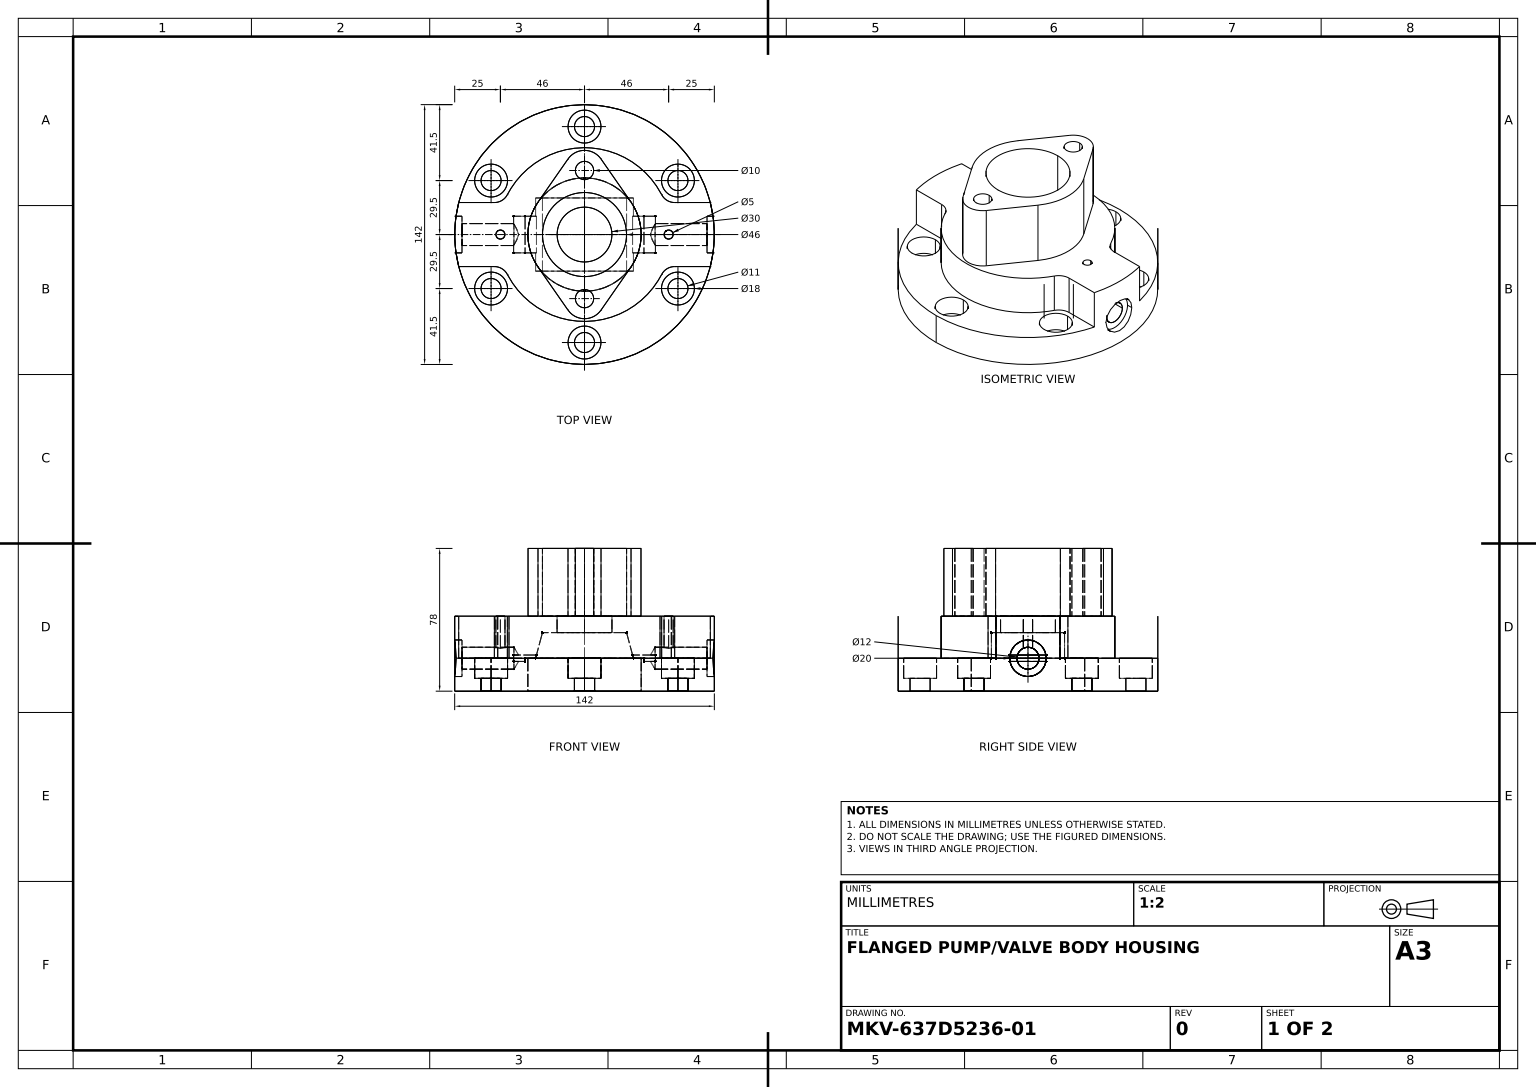
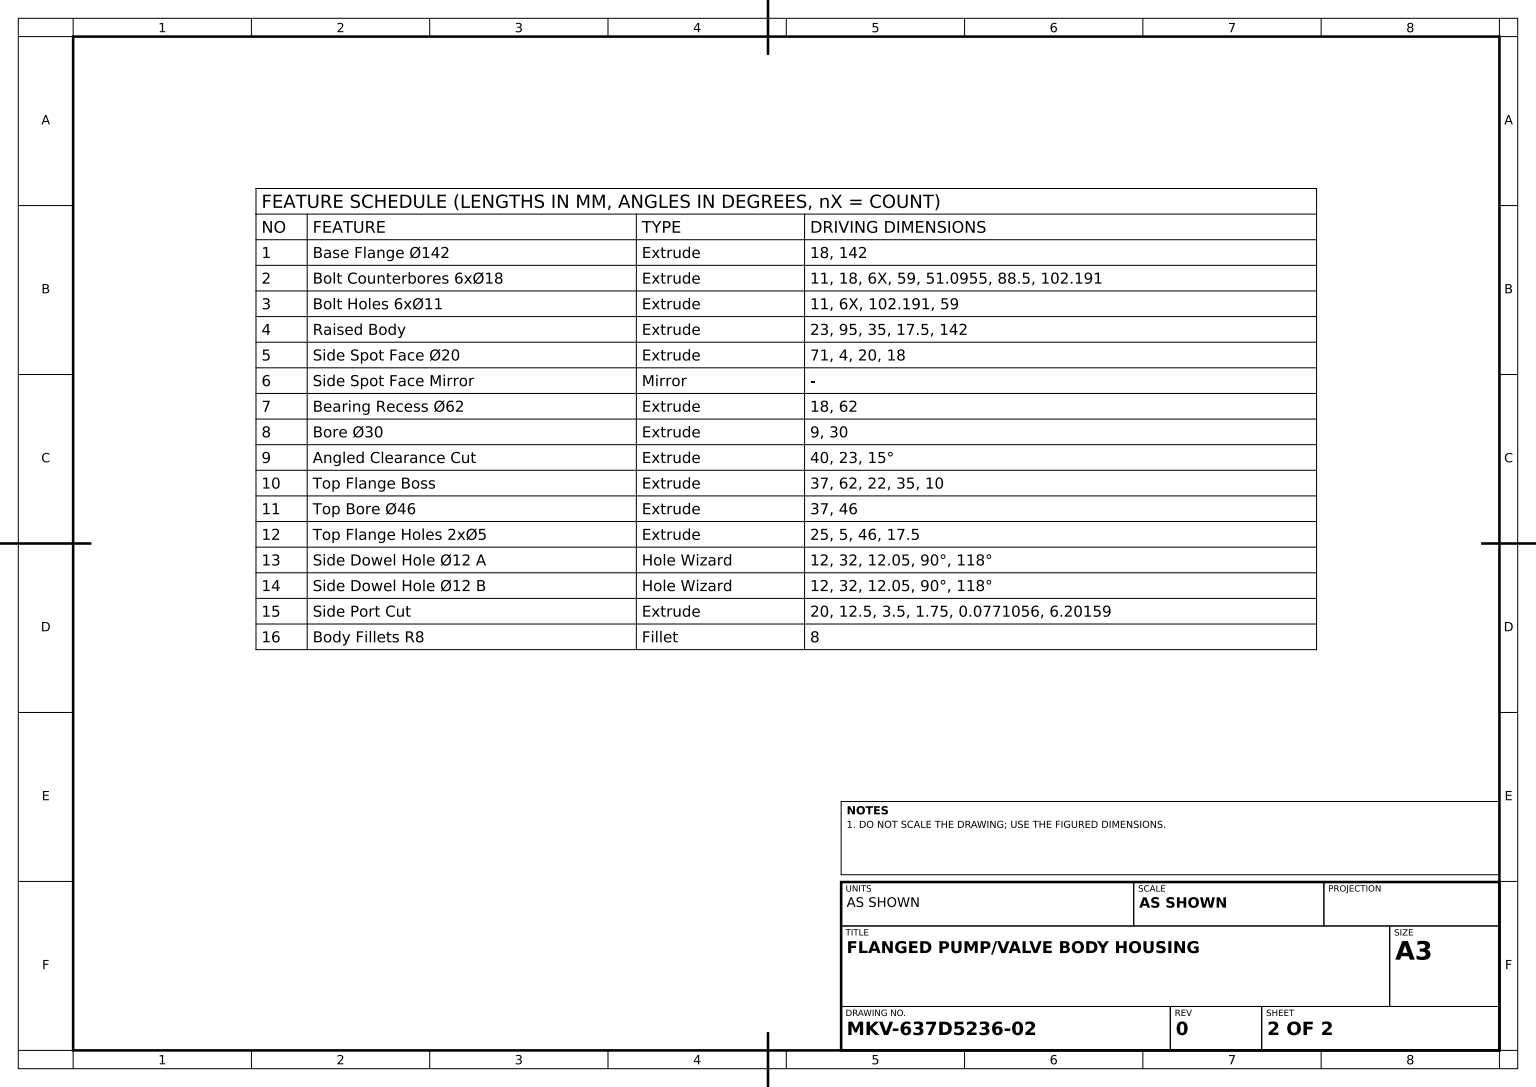
from build123d import *
from build123d.topology import SkipClean

# Parameters (mm, degrees)
BASE_FLANGE_SKETCH_R             = 71
BASE_FLANGE_142_DEPTH            = 18
COUNTERBORE_SKETCH_R             = 9
BOLT_COUNTERBORES_6X_18_DEPTH    = 11
BOLT_HOLE_SKETCH_R               = 5.5
BOLT_HOLES_6X_11_DEPTH           = 11
RAISED_BODY_DEPTH                = 23
SIDE_SPOT_FACE_SKETCH_R          = 10
SIDE_SPOT_FACE_20_DEPTH          = 4
BEARING_RECESS_SKETCH_R          = 31
BEARING_RECESS_62_DEPTH          = 18
BORE_30_SKETCH_R                 = 15
BORE_30_DEPTH                    = 9
ANGLED_CLEARANCE_CUT_DEPTH       = 20
TOP_FLANGE_BOSS_SKETCH_R         = 5
TOP_FLANGE_BOSS_DEPTH            = 37
TOP_BORE_SKETCH_R                = 23
TOP_BORE_46_DEPTH                = 37
TOP_FLANGE_HOLES_SKETCH_R        = 2.5
TOP_FLANGE_HOLES_2X_5_DEPTH      = 25
SIDE_DOWEL_HOLE_12_A_D           = 12
SIDE_DOWEL_HOLE_12_A_DEPTH       = 28.394836286
SIDE_DOWEL_HOLE_12_A_CSINK_D     = 12.05
SIDE_DOWEL_HOLE_12_A_CSINK_ANGLE = 90
SIDE_DOWEL_HOLE_12_A_TIP         = 3.605163714
SIDE_DOWEL_HOLE_12_B_D           = 12
SIDE_DOWEL_HOLE_12_B_DEPTH       = 28.394836286
SIDE_DOWEL_HOLE_12_B_CSINK_D     = 12.05
SIDE_DOWEL_HOLE_12_B_CSINK_ANGLE = 90
SIDE_DOWEL_HOLE_12_B_TIP         = 3.605163714
SIDE_PORT_CUT_DEPTH              = 10
BODY_FILLETS_R8_R                = 8


with BuildPart() as part:
    # Base Flange Sketch → Base Flange Ø142 (new body)
    with BuildSketch(Plane(origin=(0, 0, 0), x_dir=(1, 0, 0), z_dir=(0, 1, 0))):
        with Locations(Location((0, 0, 0), (0, 0, 270))):
            Circle(BASE_FLANGE_SKETCH_R)
    extrude(amount=BASE_FLANGE_142_DEPTH)

    # Counterbore Sketch → Bolt Counterbores 6xØ18 (cut)
    with BuildSketch(Plane(origin=(0, 18, 0), x_dir=(1, 0, 0), z_dir=(0, 1, 0))):
        with Locations(Location((0, 59, 0), (0, 0, 270))):
            Circle(COUNTERBORE_SKETCH_R)
        with Locations(Location((51.095498823, 29.5, 0), (0, 0, 270))):
            Circle(COUNTERBORE_SKETCH_R)
        with Locations(Location((51.095498823, -29.5, 0), (0, 0, 270))):
            Circle(COUNTERBORE_SKETCH_R)
        with Locations(Location((0, -59, 0), (0, 0, 270))):
            Circle(COUNTERBORE_SKETCH_R)
        with Locations(Location((-51.095498823, -29.5, 0), (0, 0, 270))):
            Circle(COUNTERBORE_SKETCH_R)
        with Locations(Location((-51.095498823, 29.5, 0), (0, 0, 270))):
            Circle(COUNTERBORE_SKETCH_R)
    extrude(amount=-BOLT_COUNTERBORES_6X_18_DEPTH, mode=Mode.SUBTRACT)

    # Bolt Hole Sketch → Bolt Holes 6xØ11 (cut)
    with BuildSketch(Plane(origin=(0, 7, 0), x_dir=(1, 0, 0), z_dir=(0, 1, 0))):
        with Locations(Location((-51.095498823, 29.5, 0), (0, 0, 270))):
            Circle(BOLT_HOLE_SKETCH_R)
        with Locations(Location((0, 59, 0), (0, 0, 270))):
            Circle(BOLT_HOLE_SKETCH_R)
        with Locations(Location((51.095498823, 29.5, 0), (0, 0, 270))):
            Circle(BOLT_HOLE_SKETCH_R)
        with Locations(Location((51.095498823, -29.5, 0), (0, 0, 270))):
            Circle(BOLT_HOLE_SKETCH_R)
        with Locations(Location((0, -59, 0), (0, 0, 270))):
            Circle(BOLT_HOLE_SKETCH_R)
        with Locations(Location((-51.095498823, -29.5, 0), (0, 0, 270))):
            Circle(BOLT_HOLE_SKETCH_R)
    extrude(amount=-BOLT_HOLES_6X_11_DEPTH, mode=Mode.SUBTRACT)

    # Raised Body Sketch → Raised Body (add)
    with SkipClean():  # the faces are left unmerged after this step: merging them gives an invalid solid
        with BuildSketch(Plane(origin=(0, 18, 0), x_dir=(1, 0, 0), z_dir=(0, 1, 0))):
            with BuildLine():
                Line((-68.80951969, 17.5), (-44.158804332, 17.5))
                ThreePointArc((-44.158804332, 17.5), (0, 47.5), (44.158804332, 17.5))
                Line((44.158804332, 17.5), (68.80951969, 17.5))
                ThreePointArc((68.80951969, 17.5), (71, 0), (68.80951969, -17.5))
                Line((68.80951969, -17.5), (44.158804332, -17.5))
                ThreePointArc((44.158804332, -17.5), (0, -47.5), (-44.158804332, -17.5))
                Line((-44.158804332, -17.5), (-68.80951969, -17.5))
                ThreePointArc((-68.80951969, -17.5), (-71, 0), (-68.80951969, 17.5))
            make_face()
        extrude(amount=RAISED_BODY_DEPTH)

    # Side Spot Face Sketch → Side Spot Face Ø20 (cut)
    with BuildSketch(Plane(origin=(71, 0, 0), x_dir=(0, 0, -1), z_dir=(1, 0, 0))):
        with Locations((0, 18)):
            Circle(SIDE_SPOT_FACE_SKETCH_R)
    side_spot_face_20 = extrude(amount=-SIDE_SPOT_FACE_20_DEPTH, mode=Mode.SUBTRACT)

    # Side Spot Face Mirror: Side Spot Face Ø20 across plane
    add(side_spot_face_20.mirror(Plane(origin=(0, 0, 0), x_dir=(0, 0, 1), z_dir=(1, 0, 0))), mode=Mode.SUBTRACT)

    # Bearing Recess Sketch → Bearing Recess Ø62 (cut)
    with SkipClean():  # the faces are left unmerged after this step: merging them gives an invalid solid
        with BuildSketch(Plane.XZ):
            with Locations(Location((0, 0, 0), (0, 0, 270))):
                Circle(BEARING_RECESS_SKETCH_R)
        extrude(amount=-BEARING_RECESS_62_DEPTH, mode=Mode.SUBTRACT)

    # Bore Ø30 Sketch → Bore Ø30 (cut)
    with SkipClean():  # the faces are left unmerged after this step: merging them gives an invalid solid
        with BuildSketch(Plane(origin=(0, 41, 0), x_dir=(1, 0, 0), z_dir=(0, 1, 0))):
            with Locations(Location((0, 0, 0), (0, 0, 270))):
                Circle(BORE_30_SKETCH_R)
        extrude(amount=-BORE_30_DEPTH, mode=Mode.SUBTRACT)

    # Angled Cut Sketch → Angled Clearance Cut (cut, symmetric)
    with SkipClean():  # the faces are left unmerged after this step: merging them gives an invalid solid
        with BuildSketch(Plane.XY):
            Polygon((0, 32), (23, 32), (26.751288694, 18), (-26.751288694, 18), (-23, 32), align=None)
        extrude(amount=ANGLED_CLEARANCE_CUT_DEPTH, both=True, mode=Mode.SUBTRACT)

    # Top Flange Boss Sketch → Top Flange Boss (add)
    with SkipClean():  # the faces are left unmerged after this step: merging them gives an invalid solid
        with BuildSketch(Plane(origin=(0, 41, 0), x_dir=(1, 0, 0), z_dir=(0, 1, 0))):
            with BuildLine():
                Line((-9.027169873, 41.285714286), (-25.440206006, 17.714285714))
                ThreePointArc((-25.440206006, 17.714285714), (-31, 0), (-25.440206006, -17.714285714))
                Line((-25.440206006, -17.714285714), (-9.027169873, -41.285714286))
                ThreePointArc((-9.027169873, -41.285714286), (0, -46), (9.027169873, -41.285714286))
                Line((9.027169873, -41.285714286), (25.440206006, -17.714285714))
                ThreePointArc((25.440206006, -17.714285714), (31, 0), (25.440206006, 17.714285714))
                Line((25.440206006, 17.714285714), (9.027169873, 41.285714286))
                ThreePointArc((9.027169873, 41.285714286), (0, 46), (-9.027169873, 41.285714286))
            make_face()
            with Locations(Location((0, 35, 0), (0, 0, 270))):
                Circle(TOP_FLANGE_BOSS_SKETCH_R, mode=Mode.SUBTRACT)
            with Locations(Location((0, -35, 0), (0, 0, 270))):
                Circle(TOP_FLANGE_BOSS_SKETCH_R, mode=Mode.SUBTRACT)
        extrude(amount=TOP_FLANGE_BOSS_DEPTH)

    # Top Bore Sketch → Top Bore Ø46 (cut)
    with SkipClean():  # the faces are left unmerged after this step: merging them gives an invalid solid
        with BuildSketch(Plane(origin=(0, 78, 0), x_dir=(1, 0, 0), z_dir=(0, 1, 0))):
            with Locations(Location((0, 0, 0), (0, 0, 270))):
                Circle(TOP_BORE_SKETCH_R)
        extrude(amount=-TOP_BORE_46_DEPTH, mode=Mode.SUBTRACT)

    # Top Flange Holes Sketch → Top Flange Holes 2xØ5 (cut)
    with SkipClean():  # the faces are left unmerged after this step: merging them gives an invalid solid
        with BuildSketch(Plane(origin=(0, 41, 0), x_dir=(1, 0, 0), z_dir=(0, 1, 0))):
            with Locations(Location((-46, 0, 0), (0, 0, 270))):
                Circle(TOP_FLANGE_HOLES_SKETCH_R)
            with Locations(Location((46, 0, 0), (0, 0, 270))):
                Circle(TOP_FLANGE_HOLES_SKETCH_R)
        extrude(amount=-TOP_FLANGE_HOLES_2X_5_DEPTH, mode=Mode.SUBTRACT)

    # Side Dowel Hole Ø12 A
    with Locations(Plane(origin=(67, 0, 0), x_dir=(0, 0, -1), z_dir=(1, 0, 0))):
        with Locations((0, 18)):
            CounterSinkHole(SIDE_DOWEL_HOLE_12_A_D / 2, SIDE_DOWEL_HOLE_12_A_CSINK_D / 2, depth=SIDE_DOWEL_HOLE_12_A_DEPTH, counter_sink_angle=SIDE_DOWEL_HOLE_12_A_CSINK_ANGLE)
            with Locations((0, 0, -(SIDE_DOWEL_HOLE_12_A_DEPTH + SIDE_DOWEL_HOLE_12_A_TIP / 2))):  # 118° drill point
                Cone(0, SIDE_DOWEL_HOLE_12_A_D / 2, SIDE_DOWEL_HOLE_12_A_TIP, mode=Mode.SUBTRACT)

    # Side Dowel Hole Ø12 B
    with Locations(Plane.ZY.offset(67)):
        with Locations((0, 18)):
            CounterSinkHole(SIDE_DOWEL_HOLE_12_B_D / 2, SIDE_DOWEL_HOLE_12_B_CSINK_D / 2, depth=SIDE_DOWEL_HOLE_12_B_DEPTH, counter_sink_angle=SIDE_DOWEL_HOLE_12_B_CSINK_ANGLE)
            with Locations((0, 0, -(SIDE_DOWEL_HOLE_12_B_DEPTH + SIDE_DOWEL_HOLE_12_B_TIP / 2))):  # 118° drill point
                Cone(0, SIDE_DOWEL_HOLE_12_B_D / 2, SIDE_DOWEL_HOLE_12_B_TIP, mode=Mode.SUBTRACT)

    # Side Port Sketch → Side Port Cut (cut, symmetric)
    with SkipClean():  # the faces are left unmerged after this step: merging them gives an invalid solid
        with BuildSketch(Plane.XY):
            Polygon((26.282377607, 19.75), (38.782377607, 19.75), (38.782377607, 16.25), (32.580792191, 16.25), (32.503686566, 16.25), (32.503686566, 18), (26.751288694, 18), align=None)
            Polygon((-32.503686566, 16.25), (-32.580792191, 16.25), (-38.782377607, 16.25), (-38.782377607, 19.75), (-26.282377607, 19.75), (-26.751288694, 18), (-32.503686566, 18), align=None)
        extrude(amount=SIDE_PORT_CUT_DEPTH, both=True, mode=Mode.SUBTRACT)

    # Body Fillets R8
    body_fillets_r8_edges = [part.edges().sort_by_distance(p)[0] for p in [
        (-44.158804332, 29.5, 17.5),
        (44.158804332, 29.5, 17.5),
        (44.158804332, 29.5, -17.5),
        (-44.158804332, 29.5, -17.5),
    ]]
    fillet(body_fillets_r8_edges, radius=BODY_FILLETS_R8_R)


solid = part.part
